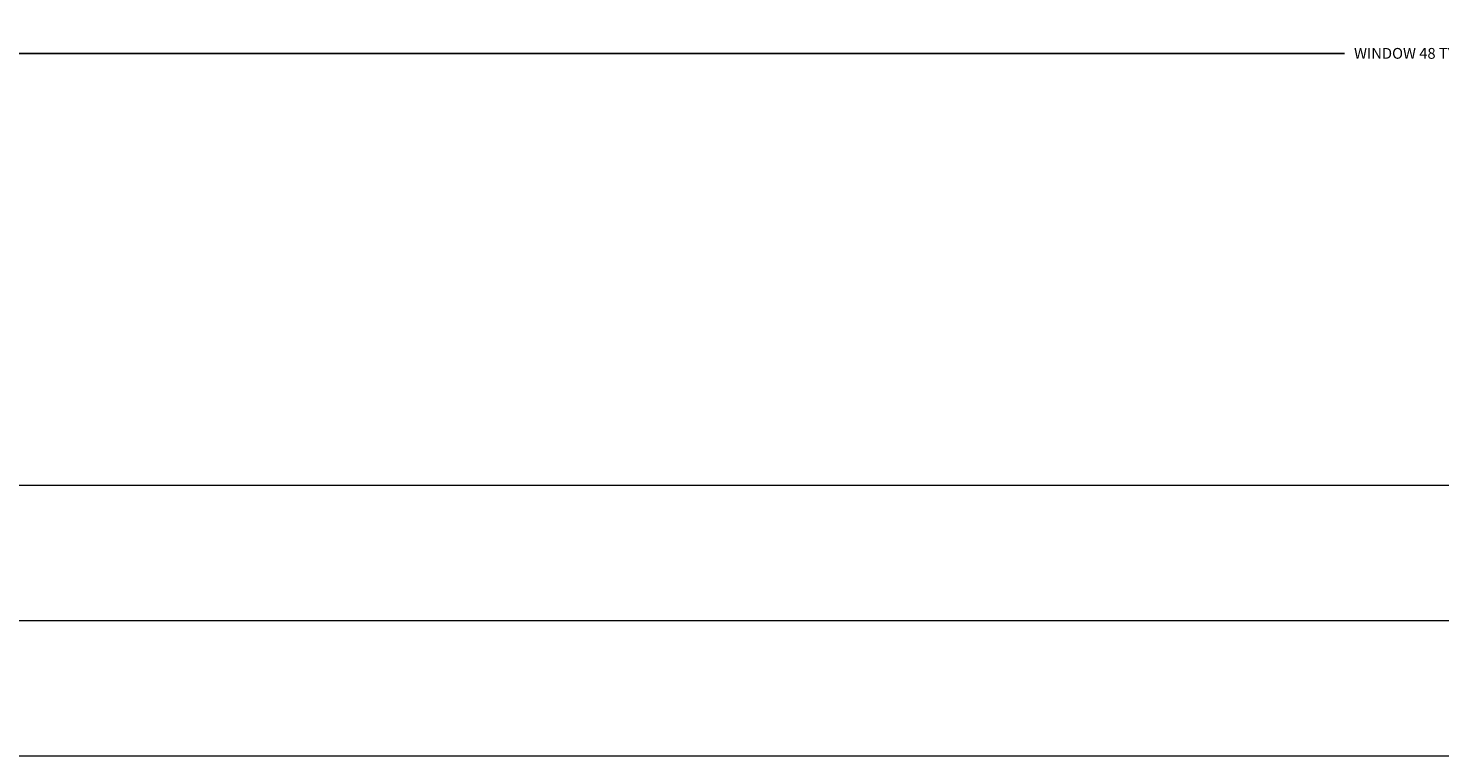
# Model space of a CAD drawing. Units: inches. Extents: x 1885 to 2748, y 783 to 2421.
# Tile 46 of 117: x 2240 to 2263, y 1558 to 1570. Entities that reach past the tile are written whole.
import ezdxf

# ---------------------------------------------------------------- set-up
doc = ezdxf.new("R2010")
doc.units = ezdxf.units.IN
doc.layers.add('A-ANNO-DIMS', color=2, linetype='Continuous', lineweight=18)
doc.layers.add('A-GLAZ', color=181, linetype='Continuous', lineweight=18)
doc.styles.get("Standard").update_dxf_attribs({"font": 'arial.ttf'})
doc.dimstyles.get("Standard").update_dxf_attribs({"dimtxt": 0.18, "dimasz": 0.18, "dimexe": 0.18, "dimexo": 0.0625, "dimgap": 0.09, "dimtad": 0, "dimtih": 1, "dimtoh": 1, "dimdec": 4, "dimzin": 0, "dimdsep": 46, "dimtxsty": 'Standard', "dimcen": 0.09, "dimadec": 0, "dimazin": 0, "dimtfac": 1, "dimtdec": 4, "dimtofl": 0, "dimtmove": 0, "dimatfit": 3, "dimfxl": 1, "dimtolj": 1, "dimtzin": 0, "dimarcsym": 0})

# ---------------------------------------------------------------- blocks, each defined once
blk = doc.blocks.new('WIN-48')
for p, q in [((48.003, 4.496), (0.003, 4.496)), ((0.003, 2.246), (48.003, 2.246)), ((0.003, -0.004), (48.003, -0.004))]:
    blk.add_line(p, q)
blk = doc.blocks.new('*D25')
at = {"layer": 'A-ANNO-DIMS', "color": 0, "lineweight": -2, "transparency": 16777216}
for p, q in [((2238.613, 1562.568), (2238.613, 1569.886)), ((2286.613, 1562.568), (2286.613, 1569.886)), ((2238.793, 1569.706), (2261.495, 1569.706)), ((2286.433, 1569.706), (2263.732, 1569.706))]:
    blk.add_line(p, q, dxfattribs=at)
at = {"layer": 'A-ANNO-DIMS', "color": 0, "transparency": 16777216}
for points in [[(2238.793, 1569.736), (2238.793, 1569.676), (2238.613, 1569.706)], [(2286.433, 1569.736), (2286.433, 1569.676), (2286.613, 1569.706)]]:
    blk.add_solid(points, dxfattribs=at)
at = {"layer": 'Defpoints', "color": 0, "transparency": 16777216}
for p in [(2286.613, 1569.706), (2238.613, 1562.506), (2286.613, 1562.506)]:
    blk.add_point(p, dxfattribs=at)
at = {"layer": 'A-ANNO-DIMS', "color": 0, "transparency": 16777216, "insert": (2262.613, 1569.706), "char_height": 0.18, "attachment_point": 5}
blk.add_mtext('\\A1;WINDOW 48 TYP.', dxfattribs=at)

msp = doc.modelspace()

# ---------------------------------------------------------------- block references
at = {"layer": 'A-GLAZ'}
msp.add_blockref('WIN-48', (2238.61, 1558.01), dxfattribs=at)

# ---------------------------------------------------------------- dimensions: what is measured, and where the dimension line sits
at = {"layer": 'A-ANNO-DIMS'}
dim = msp.add_linear_dim(base=(2286.613, 1569.706), p1=(2238.613, 1562.506), p2=(2286.613, 1562.506), text='WINDOW <> TYP.', dimstyle='Standard', override={"dimdec": 0, "dimlfac": 1, "dimrnd": 0, "dimzin": 0, "dimdsep": 46, "dimlunit": 2}, dxfattribs=at)
dim.commit()
dim.dimension.update_dxf_attribs({"geometry": '*D25', "text_midpoint": (2262.613, 1569.706)})

doc.saveas('drawing.dxf')
